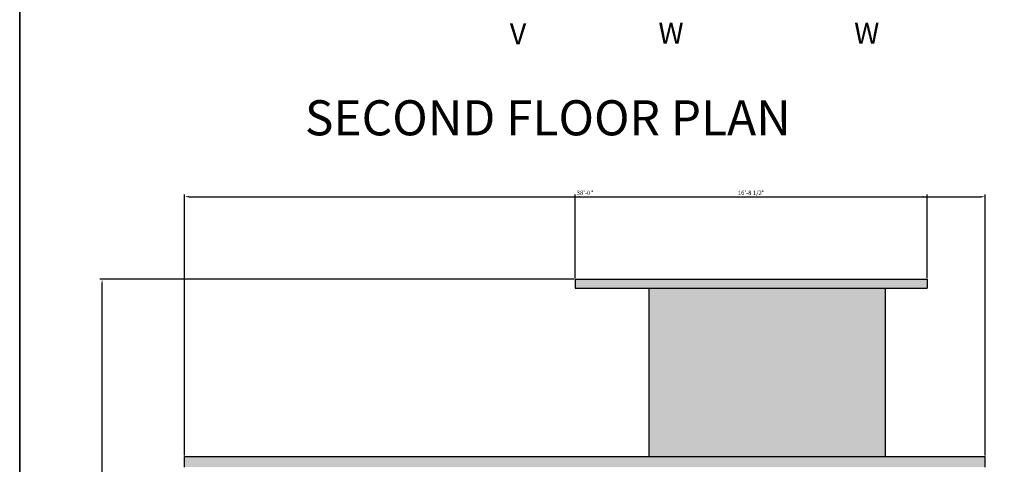
# Model space of a CAD drawing. Units: inches. Extents: x 2391 to 16591, y 7259 to 10239.
# Tile 7 of 27: x 2391 to 2952, y 8247 to 8500. Entities that reach past the tile are written whole.
import ezdxf

# ---------------------------------------------------------------- set-up
doc = ezdxf.new("R2010")
doc.units = ezdxf.units.IN
for name, color, linetype, lineweight in [('A-ANNO-DIMS', 4, 'Continuous', 18), ('A-ANNO-IDEN', 2, 'Continuous', 18), ('A-ANNO-TITL', 3, 'Continuous', 30), ('A-ANNO-TTLB', 7, 'Continuous', 35), ('A-ELEV', 7, 'Continuous', 30), ('A-ELEV-SURF-PATT', 253, 'Continuous', 13), ('A-ROOF', 7, 'Continuous', 25)]:
    doc.layers.add(name, color=color, linetype=linetype, lineweight=lineweight)
doc.styles.get("Standard").update_dxf_attribs({"font": 'arial.ttf'})
doc.dimstyles.new('ISO-25', dxfattribs={"dimtxt": 2.5, "dimasz": 2.5, "dimexe": 1.25, "dimexo": 0.625, "dimtad": 1, "dimdec": 0, "dimlunit": 3, "dimtxsty": 'Standard', "dimcen": 2.5, "dimadec": 0, "dimazin": 0, "dimtfac": 1, "dimtdec": 0, "dimtmove": 0, "dimatfit": 3, "dimfxl": 1, "dimarcsym": 0})

# ---------------------------------------------------------------- blocks, each defined once
blk = doc.blocks.new('*D78')
at = {"layer": 'A-ANNO-DIMS', "color": 0, "lineweight": -2, "transparency": 16777216}
for p, q in [((2485.26, 8251.56), (2485.26, 8400.24)), ((2487.76, 8398.99), (2938.76, 8398.99)), ((2941.26, 8251.56), (2941.26, 8400.24))]:
    blk.add_line(p, q, dxfattribs=at)
at = {"layer": 'A-ANNO-DIMS', "color": 0, "transparency": 16777216}
for points in [[(2487.76, 8399.4), (2487.76, 8398.57), (2485.26, 8398.99)], [(2938.76, 8399.4), (2938.76, 8398.57), (2941.26, 8398.99)]]:
    blk.add_solid(points, dxfattribs=at)
at = {"layer": 'Defpoints', "color": 0, "transparency": 16777216}
for p in [(2941.26, 8398.99), (2485.26, 8250.94), (2941.26, 8250.94)]:
    blk.add_point(p, dxfattribs=at)
at = {"layer": 'A-ANNO-DIMS', "color": 0, "transparency": 16777216, "insert": (2713.26, 8400.89), "char_height": 2.5, "attachment_point": 5}
blk.add_mtext('38\'-0"', dxfattribs=at)
blk = doc.blocks.new('*D79')
at = {"layer": 'A-ANNO-DIMS', "color": 0, "lineweight": -2, "transparency": 16777216}
for p, q in [((2707.14, 8351.94), (2436.96, 8351.94)), ((2438.21, 7591.44), (2438.21, 8349.44)), ((2490.64, 7588.94), (2436.96, 7588.94))]:
    blk.add_line(p, q, dxfattribs=at)
at = {"layer": 'A-ANNO-DIMS', "color": 0, "transparency": 16777216}
for points in [[(2437.8, 8349.44), (2438.63, 8349.44), (2438.21, 8351.94)], [(2437.8, 7591.44), (2438.63, 7591.44), (2438.21, 7588.94)]]:
    blk.add_solid(points, dxfattribs=at)
at = {"layer": 'Defpoints', "color": 0, "transparency": 16777216}
for p in [(2438.21, 8351.94), (2707.76, 8351.94), (2491.26, 7588.94)]:
    blk.add_point(p, dxfattribs=at)
at = {"layer": 'A-ANNO-DIMS', "color": 0, "transparency": 16777216, "insert": (2436.31, 7970.44), "char_height": 2.5, "attachment_point": 5, "rotation": 90}
blk.add_mtext('63\'-7"', dxfattribs=at)
blk = doc.blocks.new('*D82')
at = {"layer": 'A-ANNO-DIMS', "color": 0, "lineweight": -2, "transparency": 16777216}
for p, q in [((2707.76, 8352.56), (2707.76, 8400.24)), ((2710.26, 8398.99), (2905.76, 8398.99)), ((2908.26, 8352.56), (2908.26, 8400.24))]:
    blk.add_line(p, q, dxfattribs=at)
at = {"layer": 'A-ANNO-DIMS', "color": 0, "transparency": 16777216}
for points in [[(2710.26, 8399.4), (2710.26, 8398.57), (2707.76, 8398.99)], [(2905.76, 8399.4), (2905.76, 8398.57), (2908.26, 8398.99)]]:
    blk.add_solid(points, dxfattribs=at)
at = {"layer": 'Defpoints', "color": 0, "transparency": 16777216}
for p in [(2908.26, 8398.99), (2707.76, 8351.94), (2908.26, 8351.94)]:
    blk.add_point(p, dxfattribs=at)
at = {"layer": 'A-ANNO-DIMS', "color": 0, "transparency": 16777216, "insert": (2808.01, 8400.9), "char_height": 2.5, "attachment_point": 5}
blk.add_mtext('16\'-8 1/2"', dxfattribs=at)

msp = doc.modelspace()

# ---------------------------------------------------------------- hatches: boundary and pattern name
at = {"layer": 'A-ELEV-SURF-PATT'}
h = msp.add_hatch(color=256, dxfattribs=at)
h.dxf.hatch_style = 1
h.paths.add_polyline_path([(2941.26, 7764.94), (2485.26, 7764.94), (2485.26, 7758.94), (2941.26, 7758.94)])
h.paths.add_polyline_path([(2941.26, 7920.94), (2941.26, 7926.94), (2485.26, 7926.94), (2485.26, 7920.94)])
h.paths.add_polyline_path([(2941.26, 8082.94), (2941.26, 8088.94), (2485.26, 8088.94), (2485.26, 8082.94)])
h.paths.add_polyline_path([(2485.26, 8250.94), (2485.26, 8244.94), (2941.26, 8244.94), (2941.26, 8250.94)])
h.paths.add_polyline_path([(2707.76, 8351.94), (2707.76, 8346.94), (2908.26, 8346.94), (2908.26, 8351.94)])
h = msp.add_hatch(color=256, dxfattribs=at)
h.dxf.hatch_style = 1
h.paths.add_polyline_path([(2884.26, 8250.94), (2884.26, 8346.94), (2749.76, 8346.94), (2749.76, 8250.94)])

# ---------------------------------------------------------------- linework, layer by layer
at = {"layer": 'A-ANNO-TTLB'}
msp.add_lwpolyline([(2391.28, 10239.38), (4154.2, 10239.38), (4154.2, 7258.54), (2391.28, 7258.54)], close=True, dxfattribs=at)
at = {"layer": 'A-ELEV'}
for p, q in [((2485.26, 8244.94), (2485.26, 8250.94)), ((2941.26, 8244.94), (2941.26, 8250.94))]:
    msp.add_line(p, q, dxfattribs=at)
at = {"layer": 'A-ROOF'}
for p, q in [((2707.76, 8351.94), (2908.26, 8351.94)), ((2707.76, 8351.94), (2707.76, 8346.94)), ((2707.76, 8346.94), (2908.26, 8346.94)), ((2749.76, 8346.94), (2749.76, 8250.94)), ((2884.26, 8346.94), (2884.26, 8250.94)), ((2908.26, 8351.94), (2908.26, 8346.94)), ((2485.26, 8250.94), (2941.26, 8250.94))]:
    msp.add_line(p, q, dxfattribs=at)

# ---------------------------------------------------------------- texts
at = {"layer": 'A-ANNO-IDEN', "char_height": 12, "attachment_point": 1}
for s, width, insert in [('V', 46.245, (2670.46, 8497.84)), ('W', 47.6363, (2755.14, 8498.2)), ('W', 38.8857, (2866.64, 8498.14))]:
    msp.add_mtext_dynamic_manual_height_columns(s, width=width, gutter_width=12.5, heights=[0], dxfattribs=dict(at, insert=insert))
at = {"layer": 'A-ANNO-TITL', "insert": (2553.75, 8453.96), "char_height": 20, "attachment_point": 1}
msp.add_mtext_dynamic_manual_height_columns('SECOND FLOOR PLAN', width=567.8276, gutter_width=12.5, heights=[0], dxfattribs=at)

# ---------------------------------------------------------------- dimensions: what is measured, and where the dimension line sits
at = {"layer": 'A-ANNO-DIMS'}
for base, p1, p2, picture, middle in [((2941.26, 8398.99), (2485.26, 8250.94), (2941.26, 8250.94), '*D78', (2713.26, 8400.89)), ((2908.26, 8398.99), (2707.76, 8351.94), (2908.26, 8351.94), '*D82', (2808.01, 8400.9))]:
    dim = msp.add_linear_dim(base=base, p1=p1, p2=p2, dimstyle='ISO-25', override={"dimdec": 1, "dimlfac": 1, "dimrnd": 0, "dimzin": 1, "dimdsep": 46, "dimlunit": 4, "dimfrac": 2}, dxfattribs=at)
    dim.commit()
    dim.dimension.update_dxf_attribs({"geometry": picture, "text_midpoint": middle})
dim = msp.add_linear_dim(base=(2438.21, 8351.94), p1=(2491.26, 7588.94), p2=(2707.76, 8351.94), angle=90, dimstyle='ISO-25', override={"dimdec": 1, "dimlfac": 1, "dimrnd": 0, "dimzin": 1, "dimdsep": 46, "dimlunit": 4, "dimfrac": 2}, dxfattribs=at)
dim.commit()
dim.dimension.update_dxf_attribs({"geometry": '*D79', "text_midpoint": (2436.31, 7970.44)})

doc.saveas('drawing.dxf')
